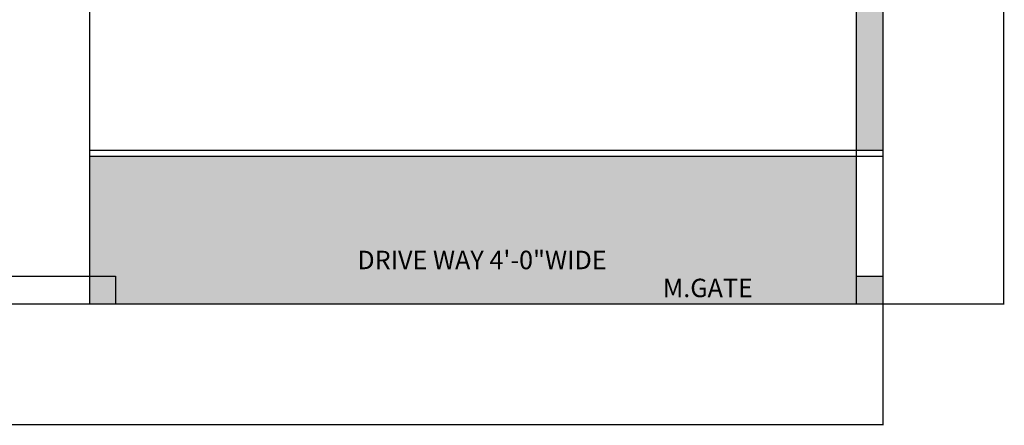
# Model space of a CAD drawing. Units: inches. Extents: x -9 to 646, y -802 to 47.
# Tile 2 of 17: x 326 to 646, y -802 to -670. Entities that reach past the tile are written whole.
import ezdxf

# ---------------------------------------------------------------- set-up
doc = ezdxf.new("R2010")
doc.units = ezdxf.units.IN
doc.header["$MEASUREMENT"] = 0
for name, color, linetype, lineweight in [('A-ANNO-DIMS', 2, 'Continuous', 18), ('A-ANNO-TEXT', 7, 'Continuous', 18), ('A-AREA-IDEN', 7, 'Continuous', 18), ('A-FLOR-PATT', 9, 'Continuous', 9), ('A-WALL-PATT', 5, 'Continuous', 9), ('C-SITE', 7, 'Continuous', 25)]:
    doc.layers.add(name, color=color, linetype=linetype, lineweight=lineweight)
doc.styles.get("Standard").update_dxf_attribs({"font": 'arial.ttf'})
doc.dimstyles.get("Standard").update_dxf_attribs({"dimtxt": 0.18, "dimasz": 0.18, "dimexe": 0.18, "dimexo": 0.0625, "dimgap": 0.09, "dimtad": 0, "dimtih": 1, "dimtoh": 1, "dimdec": 0, "dimzin": 0, "dimdsep": 46, "dimlunit": 3, "dimtxsty": 'Standard', "dimcen": 0.09, "dimadec": 0, "dimazin": 0, "dimtfac": 1, "dimtdec": 0, "dimtofl": 0, "dimtmove": 0, "dimatfit": 3, "dimfxl": 1, "dimtolj": 1, "dimtzin": 0, "dimarcsym": 0})

# ---------------------------------------------------------------- blocks, each defined once
blk = doc.blocks.new('*D49')
at = {"layer": 'A-ANNO-DIMS', "color": 0, "lineweight": -2, "transparency": 16777216}
for p, q in [((30.37, -762.13), (30.37, -801.5)), ((606.37, -762.13), (606.37, -801.5)), ((30.55, -801.32), (318.08, -801.32)), ((606.19, -801.32), (318.66, -801.32))]:
    blk.add_line(p, q, dxfattribs=at)
at = {"layer": 'A-ANNO-DIMS', "color": 0, "transparency": 16777216}
for points in [[(30.55, -801.29), (30.55, -801.35), (30.37, -801.32)], [(606.19, -801.29), (606.19, -801.35), (606.37, -801.32)]]:
    blk.add_solid(points, dxfattribs=at)
at = {"layer": 'Defpoints', "color": 0, "transparency": 16777216}
for p in [(30.37, -762.07), (606.37, -762.07), (606.37, -801.32)]:
    blk.add_point(p, dxfattribs=at)
at = {"layer": 'A-ANNO-DIMS', "color": 0, "transparency": 16777216, "insert": (318.37, -801.32), "char_height": 0.18, "attachment_point": 5}
blk.add_mtext('\\A1;576', dxfattribs=at)
blk = doc.blocks.new('*D50')
at = {"layer": 'A-ANNO-DIMS', "color": 0, "lineweight": -2, "transparency": 16777216}
for p, q in [((606.44, 7.93), (645.8, 7.93)), ((645.62, 7.75), (645.62, -376.89)), ((645.62, -761.89), (645.62, -377.25)), ((606.44, -762.07), (645.8, -762.07))]:
    blk.add_line(p, q, dxfattribs=at)
at = {"layer": 'A-ANNO-DIMS', "color": 0, "transparency": 16777216}
for points in [[(645.59, 7.75), (645.65, 7.75), (645.62, 7.93)], [(645.59, -761.89), (645.65, -761.89), (645.62, -762.07)]]:
    blk.add_solid(points, dxfattribs=at)
at = {"layer": 'Defpoints', "color": 0, "transparency": 16777216}
for p in [(606.37, 7.93), (606.37, -762.07), (645.62, -762.07)]:
    blk.add_point(p, dxfattribs=at)
at = {"layer": 'A-ANNO-DIMS', "color": 0, "transparency": 16777216, "insert": (645.62, -377.07), "char_height": 0.18, "attachment_point": 5}
blk.add_mtext('\\A1;770', dxfattribs=at)

msp = doc.modelspace()

# ---------------------------------------------------------------- hatches: boundary and pattern name
at = {"layer": 'A-FLOR-PATT'}
h = msp.add_hatch(dxfattribs=at)
h.set_pattern_fill('AR-HBONE', color=256)
h.paths.add_polyline_path([(597.63, -714.07), (348.37, -714.07), (348.37, -762.07), (597.63, -762.07)])
h.paths.add_polyline_path([(597.63, -101.57), (570.37, -101.57), (570.37, -496.07), (570.37, -511.17), (597.63, -511.17)])
at = {"layer": 'A-WALL-PATT'}
h = msp.add_hatch(color=256, dxfattribs=at)
h.dxf.hatch_style = 1
h.paths.add_polyline_path([(597.63, -101.57), (570.37, -101.57), (570.37, -496.07), (570.37, -511.17), (597.63, -511.17)], flags=0)
h.paths.add_polyline_path([(606.37, -101.57), (597.63, -101.57), (597.63, -511.17), (570.37, -511.17), (570.37, -513.2), (597.63, -513.2), (597.63, -712.07), (606.37, -712.07)])
h = msp.add_hatch(color=256, dxfattribs=at)
h.dxf.hatch_style = 1
h.paths.add_polyline_path([(356.8, -753.07), (348.37, -753.07), (348.37, -762.07), (356.8, -762.07)])
h = msp.add_hatch(color=256, dxfattribs=at)
h.dxf.hatch_style = 1
h.paths.add_polyline_path([(606.37, -753.07), (597.63, -753.07), (597.63, -762.07), (606.37, -762.07)])

# ---------------------------------------------------------------- linework, layer by layer
at = {"layer": 'C-SITE'}
for p, q in [((606.37, -101.57), (606.37, -762.07)), ((597.63, -513.2), (597.63, -762.07)), ((348.37, -646.07), (348.37, -762.07)), ((348.37, -712.07), (606.37, -712.07)), ((348.37, -714.07), (606.37, -714.07)), ((39.59, -753.07), (348.37, -753.07)), ((348.37, -753.07), (356.8, -753.07)), ((356.8, -753.07), (356.8, -762.07)), ((597.63, -753.07), (606.37, -753.07)), ((30.37, -762.07), (606.37, -762.07))]:
    msp.add_line(p, q, dxfattribs=at)

# ---------------------------------------------------------------- texts
at = {"layer": 'A-ANNO-TEXT', "insert": (534.79, -753.86), "char_height": 6, "attachment_point": 1}
msp.add_mtext('M.GATE', dxfattribs=at)
at = {"layer": 'A-AREA-IDEN', "insert": (435.46, -744.77), "char_height": 6, "attachment_point": 1}
msp.add_mtext('DRIVE WAY 4\'-0"WIDE', dxfattribs=at)

# ---------------------------------------------------------------- dimensions: what is measured, and where the dimension line sits
at = {"layer": 'A-ANNO-DIMS'}
dim = msp.add_linear_dim(base=(645.62, -762.07), p1=(606.37, 7.93), p2=(606.37, -762.07), angle=90, dimstyle='Standard', override={"dimdec": 0, "dimlfac": 1, "dimrnd": 0, "dimzin": 0, "dimdsep": 46, "dimlunit": 2}, dxfattribs=at)
dim.commit()
dim.dimension.update_dxf_attribs({"geometry": '*D50', "text_midpoint": (645.62, -377.07)})
dim = msp.add_linear_dim(base=(606.37, -801.32), p1=(30.37, -762.07), p2=(606.37, -762.07), dimstyle='Standard', override={"dimdec": 0, "dimlfac": 1, "dimrnd": 0, "dimzin": 0, "dimdsep": 46, "dimlunit": 2}, dxfattribs=at)
dim.commit()
dim.dimension.update_dxf_attribs({"geometry": '*D49', "text_midpoint": (318.37, -801.32)})

doc.saveas('drawing.dxf')
